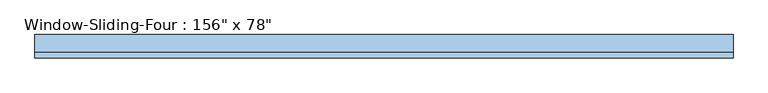
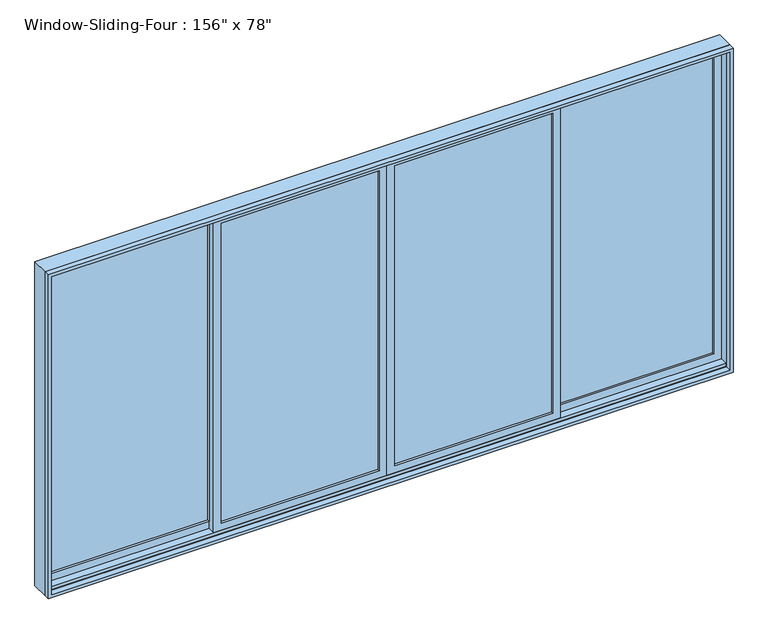
"""IFC4 building model written with IfcOpenShell, lengths in millimetres: window geometry."""

from ifc_helpers import new_model, si_unit, frame, origin, place, context, project, spatial, polyline, outline, extrude, faceted_brep, source, transform, mapped, element, save


def window_cbca41e3(model_context):
    return source(origin(), model_context, "Body", "SolidModel", [
        extrude(outline(polyline([(933.45, -1962.15), (933.45, -958.85), (2876.55, -958.85), (2876.55, -1962.15), (933.45, -1962.15)]), holes=[polyline([(2832.1, -1003.3), (996.95, -1003.3), (996.95, -1917.7), (2832.1, -1917.7), (2832.1, -1003.3)])]), frame((0.0, 21.59, 0.0), z_axis=(0.0, 1.0, 0.0), x_axis=(0.0, 0.0, 1.0)), (0.0, 0.0, 1.0), 44.45),
        extrude(outline(polyline([(-1003.3, 53.34), (-1003.3, 46.99), (-1917.7, 46.99), (-1917.7, 53.34), (-1003.3, 53.34)])), frame((0.0, 0.0, 996.95), z_axis=(0.0, 0.0, 1.0), x_axis=(1.0, 0.0, 0.0)), (0.0, 0.0, 1.0), 1835.15),
        extrude(outline(polyline([(-1003.3, 40.64), (-1003.3, 34.29), (-1917.7, 34.29), (-1917.7, 40.64), (-1003.3, 40.64)])), frame((0.0, 0.0, 996.95), z_axis=(0.0, 0.0, 1.0), x_axis=(1.0, 0.0, 0.0)), (0.0, 0.0, 1.0), 1835.15),
        extrude(outline(polyline([(-44.45, 8.89), (-44.45, 2.54), (-958.85, 2.54), (-958.85, 8.89), (-44.45, 8.89)])), frame((0.0, 0.0, 996.95), z_axis=(0.0, 0.0, 1.0), x_axis=(1.0, 0.0, 0.0)), (0.0, 0.0, 1.0), 1835.15),
        extrude(outline(polyline([(-44.45, -3.81), (-44.45, -10.16), (-958.85, -10.16), (-958.85, -3.81), (-44.45, -3.81)])), frame((0.0, 0.0, 996.95), z_axis=(0.0, 0.0, 1.0), x_axis=(1.0, 0.0, 0.0)), (0.0, 0.0, 1.0), 1835.15),
        extrude(outline(polyline([(2895.6, -1981.2), (914.4, -1981.2), (914.4, 1981.2), (2895.6, 1981.2), (2895.6, -1981.2)]), holes=[polyline([(2876.55, 1962.15), (933.45, 1962.15), (933.45, -1962.15), (2876.55, -1962.15), (2876.55, 1962.15)])]), frame((0.0, -60.96, 0.0), z_axis=(0.0, 1.0, 0.0), x_axis=(0.0, 0.0, 1.0)), (0.0, 0.0, 1.0), 31.75),
        extrude(outline(polyline([(952.5, 1003.3), (2876.55, 1003.3), (2876.55, 0.0), (952.5, 0.0), (952.5, 1003.3)]), holes=[polyline([(996.95, 44.45), (2832.1, 44.45), (2832.1, 958.85), (996.95, 958.85), (996.95, 44.45)])]), frame((0.0, -22.86, 0.0), z_axis=(0.0, 1.0, 0.0), x_axis=(0.0, 0.0, 1.0)), (0.0, 0.0, 1.0), 44.45),
        extrude(outline(polyline([(2876.55, -1003.3), (952.5, -1003.3), (952.5, 0.0), (2876.55, 0.0), (2876.55, -1003.3)]), holes=[polyline([(2832.1, -44.45), (996.95, -44.45), (996.95, -958.85), (2832.1, -958.85), (2832.1, -44.45)])]), frame((0.0, -22.86, 0.0), z_axis=(0.0, 1.0, 0.0), x_axis=(0.0, 0.0, 1.0)), (0.0, 0.0, 1.0), 44.45),
        extrude(outline(polyline([(958.85, 8.89), (958.85, 2.54), (44.45, 2.54), (44.45, 8.89), (958.85, 8.89)])), frame((0.0, 0.0, 996.95), z_axis=(0.0, 0.0, 1.0), x_axis=(1.0, 0.0, 0.0)), (0.0, 0.0, 1.0), 1835.15),
        extrude(outline(polyline([(958.85, -3.81), (958.85, -10.16), (44.45, -10.16), (44.45, -3.81), (958.85, -3.81)])), frame((0.0, 0.0, 996.95), z_axis=(0.0, 0.0, 1.0), x_axis=(1.0, 0.0, 0.0)), (0.0, 0.0, 1.0), 1835.15),
        extrude(outline(polyline([(1917.7, 53.34), (1917.7, 46.99), (1003.3, 46.99), (1003.3, 53.34), (1917.7, 53.34)])), frame((0.0, 0.0, 996.95), z_axis=(0.0, 0.0, 1.0), x_axis=(1.0, 0.0, 0.0)), (0.0, 0.0, 1.0), 1835.15),
        extrude(outline(polyline([(1917.7, 40.3225303), (1917.7, 34.29), (1003.3, 34.29), (1003.3, 40.3225303), (1917.7, 40.3225303)])), frame((0.0, 0.0, 996.95), z_axis=(0.0, 0.0, 1.0), x_axis=(1.0, 0.0, 0.0)), (0.0, 0.0, 1.0), 1835.15),
        extrude(outline(polyline([(933.45, 1962.15), (2876.55, 1962.15), (2876.55, 958.85), (933.45, 958.85), (933.45, 1962.15)]), holes=[polyline([(2832.1, 1003.3), (2832.1, 1917.7), (996.95, 1917.7), (996.95, 1003.3), (2832.1, 1003.3)])]), frame((0.0, 21.59, 0.0), z_axis=(0.0, 1.0, 0.0), x_axis=(0.0, 0.0, 1.0)), (0.0, 0.0, 1.0), 44.45),
        faceted_brep([(-1981.2, -29.21, 914.4), (-1981.2, 72.39, 914.4), (1981.2, 72.39, 914.4), (1981.2, -29.21, 914.4), (-1940.2778905, 72.39, 2854.6778905), (-1940.2778905, 66.04, 2854.6778905), (-1940.2778905, 66.04, 933.45), (-1940.2778905, 72.39, 933.45), (1940.2778905, 66.04, 2854.6778905), (1940.2778905, 66.04, 933.45), (1962.15, 66.04, 933.45), (1962.15, 66.04, 2876.55), (-1962.15, 66.04, 2876.55), (-1962.15, 66.04, 933.45), (-1962.15, -29.21, 2876.55), (-1962.15, -29.21, 933.45), (-1962.15, -22.86, 933.45), (-1962.15, -22.86, 952.5), (-1962.15, 21.59, 952.5), (-1962.15, 21.59, 933.45), (1981.2, -29.21, 2895.6), (-1981.2, -29.21, 2895.6), (1962.15, -29.21, 2876.55), (1962.15, -29.21, 933.45), (-1981.2, 72.39, 2895.6), (1981.2, 72.39, 2895.6), (1940.2778905, 72.39, 933.45), (1940.2778905, 72.39, 2854.6778905), (1962.15, 21.59, 933.45), (1962.15, 21.59, 952.5), (1962.15, -22.86, 952.5), (1962.15, -22.86, 933.45)], [[[0, 1, 2, 3]], [[4, 5, 6, 7]], [[5, 8, 9, 10, 11, 12, 13, 6]], [[12, 14, 15, 16, 17, 18, 19, 13]], [[0, 3, 20, 21], [22, 23, 15, 14]], [[24, 1, 0, 21]], [[2, 1, 24, 25], [4, 7, 26, 27]], [[5, 4, 27, 8]], [[12, 11, 22, 14]], [[21, 20, 25, 24]], [[8, 27, 26, 9]], [[22, 11, 10, 28, 29, 30, 31, 23]], [[20, 3, 2, 25]], [[26, 7, 6, 13, 19, 28, 10, 9]], [[28, 19, 18, 29]], [[29, 18, 17, 30]], [[30, 17, 16, 31]], [[15, 23, 31, 16]]]),
    ])


if __name__ == "__main__":
    model = new_model("IFC4")
    model_context = context("Model", 3, world=origin())
    ifc_project = project(units=[si_unit("LENGTHUNIT", "METRE", prefix="MILLI")], contexts=[model_context])
    site = spatial("IfcSite", under=ifc_project)
    building = spatial("IfcBuilding", under=site)
    placement = place(None, origin())
    window_shape = window_cbca41e3(model_context)
    element("IfcWindow", 1, ObjectType="Window-Sliding-Four : 156\" x 78\"", at=placement, inside=building, context=model_context, shape_type="MappedRepresentation", body=[
        mapped(window_shape, transform((0.0, 0.0, 0.0), x_axis=(1.0, 0.0, 0.0), y_axis=(0.0, 1.0, 0.0), z_axis=(0.0, 0.0, 1.0))),
    ])
    save(model, "model.ifc")

# Revit data of these elements
# Type "Window-Sliding-Four : 156\" x 78\""
#   Type Mark = "21"
#   Fire Rating = "0.5h"
#   Assembly Code = "B2020100"
#   Analytic Construction = "Double glazing - domestic"
#   Window Inset [instance default] = 0 ft
#   Wall Thickness [instance default] = 0.5 ft
#   Visual Light Transmittance = 0.81
#   Thermal Resistance (R) = 1.8146 (h·ft²·°F)/BTU
#   Solar Heat Gain Coefficient = 0.76
#   Interior Wall Closure [instance default] = 0.216146 ft
#   Heat Transfer Coefficient (U) = 0.5511 BTU/(h·ft²·°F)
#   Frame Extension [instance default] = 0.020833 ft
#   Exterior Wall Closure [instance default] = 0.104167 ft
#   Rough Width = 13.041667 ft
#   Rough Height = 6.541667 ft
#   Height = 6.5 ft
#   Extension Jamb [instance default] = 0.229167 ft
#   Default Sill Height = 3 ft
#   Width = 13 ft
#   Middle Muntin Visibility = yes
#   Interior Trim Visibility [instance default] = yes
#   Indicator Visibility [instance default] = yes
#   Exterior Trim Visibility [instance default] = yes
#   Side Muntin Visibility = yes
#   Extension Jamb Visibility [instance default] = yes
#   Interior Trim Material = Wood - Stained
#   Muntin Pattern = Muntin Pattern_2x2 : Muntin Pattern_2x2
#   Interior Trim = Trim-Window-Interior-Flat : Picture Frame
#   Interior Frame Material = Wood - Stained
#   Glass Panel Material = Glass
#   Exterior Trim Material = Clad - White
#   Exterior Trim = Trim-Window-Exterior-Flat : with Sill
#   Exterior Frame Material = Clad - White
#   Wall Closure = (empty or 0)
# Element 1 (IfcWindow, "Window-Sliding-Four : 156\" x 78\"")
#   Wall Thickness = 0.375 ft
#   Extension Jamb = 0.104167 ft
#   Materials on its faces: "Wood - Stained", "Glass", "Clad - White"
# Materials
#   "Wood - Stained": class "Wood", colour RGB 224 178 126, transparency 0, Cost = 0
#   "Glass": class "Glass", colour RGB 0 128 192, transparency 0.75, Description = "Soda Lime Glass", Cost = 0
#   "Clad - White": class "Wood", colour RGB 242 242 238, transparency 0, Cost = 0
